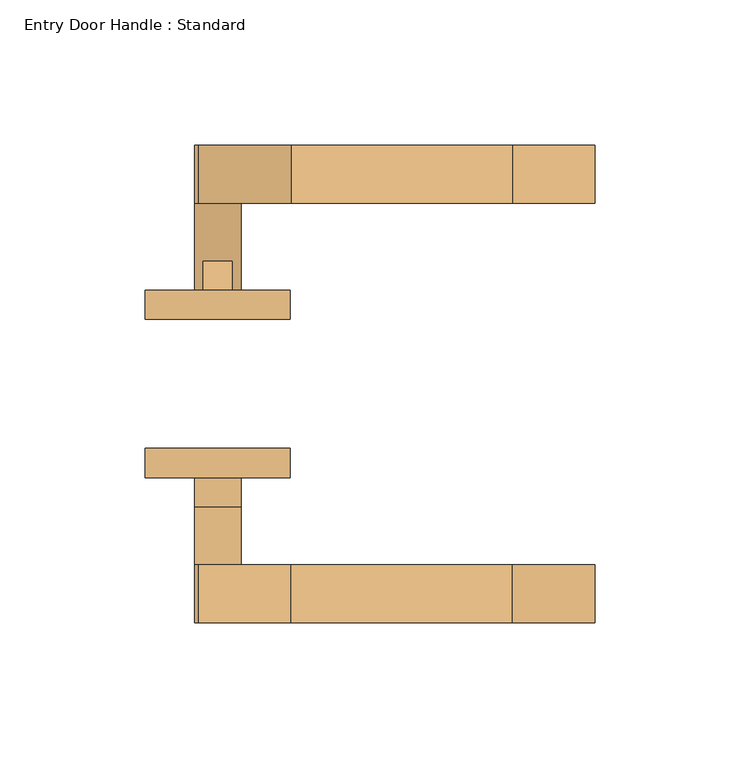
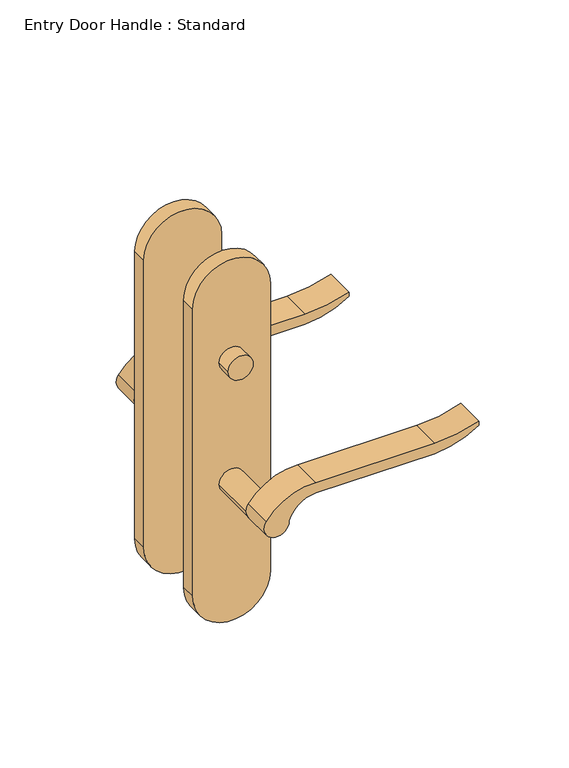
"""IFC4 building model written with IfcOpenShell, lengths in millimetres: door geometry, Entry Door Handle : Standard."""

from ifc_helpers import new_model, si_unit, point, frame, frame_2d, origin, origin_2d, place, context, project, spatial, polyline, circle_curve, trimmed, segment, composite_curve, outline, extrude, source, transform, mapped, element, save


def entry_door_handle_standard_87575fd4(model_context):
    return source(origin(), model_context, "Body", "SweptSolid", [
        extrude(outline(polyline([(-5.0, 42.225), (5.0, 42.225), (5.0, 32.225), (-5.0, 32.225), (-5.0, 42.225)])), frame((0.0, 0.0, 67.5), z_axis=(0.0, 0.0, 1.0), x_axis=(1.0, 0.0, 0.0)), (0.0, 0.0, 1.0), 30.0),
        extrude(outline(composite_curve([segment(trimmed(circle_curve(frame_2d((82.5, 0.0)), 8.0), [point((82.5, 8.0))], [point((82.5, -8.0))], False, "CARTESIAN"), True, "CONTINUOUS"), segment(trimmed(circle_curve(frame_2d((82.5, 0.0)), 8.0), [point((82.5, -8.0))], [point((82.5, 8.0))], False, "CARTESIAN"), True, "CONTINUOUS")], self_intersect=False)), frame((0.0, -42.225, 0.0), z_axis=(0.0, 1.0, 0.0), x_axis=(0.0, 0.0, 1.0)), (0.0, 0.0, 1.0), 10.0),
        extrude(outline(composite_curve([segment(trimmed(circle_curve(origin_2d(), 8.0), [point((4.6523287, -6.5081363))], [point((0.0, 8.0))], False, "CARTESIAN"), True, "CONTINUOUS"), segment(trimmed(circle_curve(frame_2d((-5.1261387, 25.3861901)), 18.1261387), [point((0.0, 8.0))], [point((13.0, 25.3861901))], True, "CARTESIAN"), True, "CONTINUOUS"), segment(polyline([(13.0, 25.3861901), (13.0, 101.6435909)]), True, "CONTINUOUS"), segment(trimmed(circle_curve(frame_2d((72.2709207, 98.0603388)), 59.3791355), [point((13.0, 101.6435909))], [point((22.2135558, 130.0))], False, "CARTESIAN"), True, "CONTINUOUS"), segment(polyline([(22.2135558, 130.0), (25.0, 130.0)]), True, "CONTINUOUS"), segment(trimmed(circle_curve(frame_2d((103.2850638, 101.5772091)), 83.2850902), [point((25.0, 130.0))], [point((20.0, 101.6435909))], True, "CARTESIAN"), True, "CONTINUOUS"), segment(polyline([(20.0, 101.6435909), (20.0, 25.3674333)]), True, "CONTINUOUS"), segment(trimmed(circle_curve(frame_2d((-17.2444479, 23.6675129)), 37.2832219), [point((20.0, 25.3674333))], [point((4.6523287, -6.5081363))], False, "CARTESIAN"), True, "CONTINUOUS")], self_intersect=False)), frame((0.0, 62.225, 0.0), z_axis=(0.0, 1.0, 0.0), x_axis=(0.0, 0.0, 1.0)), (0.0, 0.0, 1.0), 20.0),
        extrude(outline(composite_curve([segment(trimmed(circle_curve(frame_2d((-5.1261318, 25.3861878)), 18.1261318), [point((-9.7e-06, 8.0))], [point((13.0, 25.3861878))], True, "CARTESIAN"), True, "CONTINUOUS"), segment(polyline([(13.0, 25.3861878), (13.0, 101.6435909)]), True, "CONTINUOUS"), segment(trimmed(circle_curve(frame_2d((72.2709207, 98.0603388)), 59.3791355), [point((13.0, 101.6435909))], [point((22.2135558, 130.0))], False, "CARTESIAN"), True, "CONTINUOUS"), segment(polyline([(22.2135558, 130.0), (25.0, 130.0)]), True, "CONTINUOUS"), segment(trimmed(circle_curve(frame_2d((103.2850638, 101.5772091)), 83.2850902), [point((25.0, 130.0))], [point((20.0, 101.6435909))], True, "CARTESIAN"), True, "CONTINUOUS"), segment(polyline([(20.0, 101.6435909), (20.0, 25.3674333)]), True, "CONTINUOUS"), segment(trimmed(circle_curve(frame_2d((-17.2444479, 23.6675129)), 37.2832219), [point((20.0, 25.3674333))], [point((4.6523287, -6.5081363))], False, "CARTESIAN"), True, "CONTINUOUS"), segment(trimmed(circle_curve(origin_2d(), 8.0), [point((4.6523287, -6.5081363))], [point((-9.7e-06, 8.0))], False, "CARTESIAN"), True, "CONTINUOUS")], self_intersect=False)), frame((0.0, -82.225, 0.0), z_axis=(0.0, 1.0, 0.0), x_axis=(0.0, 0.0, 1.0)), (0.0, 0.0, 1.0), 20.0),
        extrude(outline(composite_curve([segment(trimmed(circle_curve(origin_2d(), 8.0), [point((0.0, 8.0))], [point((0.0, -8.0))], False, "CARTESIAN"), True, "CONTINUOUS"), segment(trimmed(circle_curve(origin_2d(), 8.0), [point((0.0, -8.0))], [point((0.0, 8.0))], False, "CARTESIAN"), True, "CONTINUOUS")], self_intersect=False)), frame((0.0, 32.225, 0.0), z_axis=(0.0, 1.0, 0.0), x_axis=(0.0, 0.0, 1.0)), (0.0, 0.0, 1.0), 30.0),
        extrude(outline(composite_curve([segment(trimmed(circle_curve(origin_2d(), 8.0), [point((0.0, 8.0))], [point((0.0, -8.0))], False, "CARTESIAN"), True, "CONTINUOUS"), segment(trimmed(circle_curve(origin_2d(), 8.0), [point((0.0, -8.0))], [point((0.0, 8.0))], False, "CARTESIAN"), True, "CONTINUOUS")], self_intersect=False)), frame((0.0, -62.225, 0.0), z_axis=(0.0, 1.0, 0.0), x_axis=(0.0, 0.0, 1.0)), (0.0, 0.0, 1.0), 30.0),
        extrude(outline(composite_curve([segment(trimmed(circle_curve(frame_2d((-70.0, 0.0)), 25.0), [point((-70.0, -25.0))], [point((-70.0, 25.0))], False, "CARTESIAN"), True, "CONTINUOUS"), segment(polyline([(-70.0, 25.0), (125.0, 25.0)]), True, "CONTINUOUS"), segment(trimmed(circle_curve(frame_2d((125.0, 0.0)), 25.0), [point((125.0, 25.0))], [point((125.0, -25.0))], False, "CARTESIAN"), True, "CONTINUOUS"), segment(polyline([(125.0, -25.0), (-70.0, -25.0)]), True, "CONTINUOUS")], self_intersect=False)), frame((0.0, 22.225, 0.0), z_axis=(0.0, 1.0, 0.0), x_axis=(0.0, 0.0, 1.0)), (0.0, 0.0, 1.0), 10.0),
        extrude(outline(composite_curve([segment(trimmed(circle_curve(frame_2d((-70.0, 0.0)), 25.0), [point((-70.0, -25.0))], [point((-70.0, 25.0))], False, "CARTESIAN"), True, "CONTINUOUS"), segment(polyline([(-70.0, 25.0), (125.0, 25.0)]), True, "CONTINUOUS"), segment(trimmed(circle_curve(frame_2d((125.0, 0.0)), 25.0), [point((125.0, 25.0))], [point((125.0, -25.0))], False, "CARTESIAN"), True, "CONTINUOUS"), segment(polyline([(125.0, -25.0), (-70.0, -25.0)]), True, "CONTINUOUS")], self_intersect=False)), frame((0.0, -32.225, 0.0), z_axis=(0.0, 1.0, 0.0), x_axis=(0.0, 0.0, 1.0)), (0.0, 0.0, 1.0), 10.0),
    ])


if __name__ == "__main__":
    model = new_model("IFC4")
    model_context = context("Model", 3, world=origin())
    ifc_project = project(units=[si_unit("LENGTHUNIT", "METRE", prefix="MILLI")], contexts=[model_context])
    site = spatial("IfcSite", under=ifc_project)
    building = spatial("IfcBuilding", under=site)
    placement = place(None, origin())
    entry_door_handle_standard_shape = entry_door_handle_standard_87575fd4(model_context)
    element("IfcDoor", 1, ObjectType="Entry Door Handle : Standard", at=placement, inside=building, context=model_context, shape_type="MappedRepresentation", body=[
        mapped(entry_door_handle_standard_shape, transform((0.0, 0.0, 0.0), x_axis=(1.0, 0.0, 0.0), y_axis=(0.0, 1.0, 0.0), z_axis=(0.0, 0.0, 1.0))),
    ])
    save(model, "model.ifc")

# Revit data of these elements
# Type "Entry Door Handle : Standard"
#   Type Mark = "10"
#   Analytic Construction = "<None>"
#   Thickness = 0' - 1 3/4"
#   Handle Material = Aluminum
#   Function = (empty or 0)
#   Construction Type = (empty or 0)
# Element 1 (IfcDoor, "Entry Door Handle : Standard")
#   Materials on its faces: "Aluminum"
# Materials
#   "Aluminum": class "Metal", colour RGB 247 247 247, transparency 0, Description = "Aluminum 6061", Cost = 0
